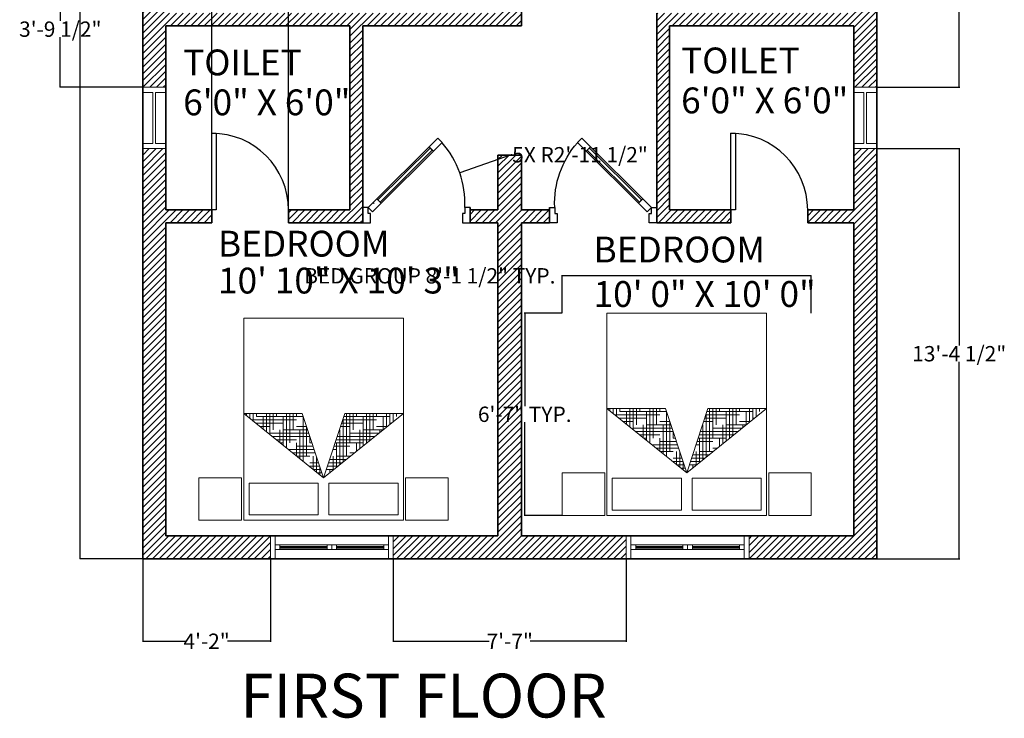
# Model space of a CAD drawing. Units: inches. Extents: x 585 to 1401, y -184 to 463.
# Tile 7 of 8: x 1016 to 1401, y -172 to 101. Entities that reach past the tile are written whole.
import ezdxf

# ---------------------------------------------------------------- set-up
doc = ezdxf.new("R2010")
doc.units = ezdxf.units.IN
doc.header["$MEASUREMENT"] = 0
for name, color, linetype, lineweight in [('A-ANNO-DIMS', 2, 'Continuous', 18), ('A-ANNO-TEXT', 7, 'Continuous', 25), ('A-AREA-IDEN', 7, 'Continuous', 18), ('A-Door', 150, 'Continuous', 25), ('A-FURN', 8, 'Continuous', 18), ('A-Glaz', 140, 'Continuous', 18), ('A-Wall', 7, 'Continuous', 35), ('A-WALL-PATT', 252, 'Continuous', 13)]:
    doc.layers.add(name, color=color, linetype=linetype, lineweight=lineweight)
doc.styles.get("Standard").update_dxf_attribs({"font": 'arial.ttf'})
doc.dimstyles.get("Standard").update_dxf_attribs({"dimtxt": 6, "dimasz": 0.18, "dimexe": 0.18, "dimexo": 0.0625, "dimgap": 0.09, "dimtad": 0, "dimtih": 1, "dimtoh": 1, "dimdec": 0, "dimzin": 0, "dimdsep": 46, "dimlunit": 3, "dimtxsty": 'Standard', "dimblk": 'ARCHTICK', "dimcen": 0.09, "dimadec": 0, "dimazin": 0, "dimtfac": 1, "dimtdec": 0, "dimtofl": 0, "dimtmove": 0, "dimatfit": 3, "dimfxl": 1, "dimtolj": 1, "dimtzin": 0, "dimarcsym": 0})

# ---------------------------------------------------------------- blocks, each defined once
blk = doc.blocks.new('A$C1DF4181C')
blk.add_lwpolyline([(120, 128), (460.7, 466.1), (432.5, 494.5), (91.8, 156.4)], close=True)
blk.add_arc((72.4, 128.7), 593.3, 357.23132, 41.49368)
at = {"layer": 'A-Door'}
for points in [[(517.5, 522.4), (460.7, 466.1), (432.5, 494.5), (489.3, 550.8)], [(63.2, 71.6), (120, 128), (91.8, 156.4), (35, 100)], [(35, 100), (0, 100), (0, 0), (50, 0), (50, 50), (50, 60), (35, 60)], [(665, 100), (665, 60), (650, 60), (650, 50), (650, 0), (700, 0), (700, 100)]]:
    blk.add_lwpolyline(points, close=True, dxfattribs=at)
at = {"layer": 'A-Glaz'}
blk.add_lwpolyline([(112.9, 135.1), (453.6, 473.2), (439.5, 487.4), (98.8, 149.3)], close=True, dxfattribs=at)
at = {"layer": 'A-Wall'}
for p, q in [((0, 0), (0, 100)), ((0, 100), (0, 0)), ((700, 0), (700, 100)), ((700, 0), (700, 100))]:
    blk.add_line(p, q, dxfattribs=at)
blk = doc.blocks.new('*U9')
for p, q in [((0, 0), (0, -5)), ((30, 0), (30, -5))]:
    blk.add_line(p, q)
blk.add_lwpolyline([(0, 0), (0, 30), (1.75, 30), (1.75, 0)], close=True)
blk.add_arc((0, 0), 30, 0, 90)
blk = doc.blocks.new('*X23')
at = {"color": 0}
for p, q in [((20.25, 14.8125), (20.2772, 14.8125)), ((20.1487, 14.7188), (20.2772, 14.7188)), ((20.1562, 14.625), (20.1562, 14.7281)), ((20.1739, 14.75), (20.2772, 14.75)), ((20.1875, 14.75), (20.1875, 14.7669)), ((20.199, 14.7812), (20.2772, 14.7812)), ((20.25, 14.3194), (20.25, 14.75)), ((20.0625, 14.2573), (20.0625, 14.6116)), ((20.0938, 14.375), (20.0938, 14.6504)), ((20.0984, 14.6562), (20.125, 14.6562)), ((20.1236, 14.6875), (20.25, 14.6875)), ((20.125, 14.5), (20.125, 14.6893)), ((20.2188, 14.3091), (20.2188, 14.625)), ((20.25, 14.625), (20.2772, 14.625)), ((19.9979, 14.5312), (20.2772, 14.5312)), ((20.023, 14.5625), (20.2772, 14.5625)), ((20.0312, 14.2469), (20.0312, 14.5727)), ((20.125, 14.5938), (20.2772, 14.5938)), ((19.9225, 14.4375), (20, 14.4375)), ((19.9476, 14.4688), (20.125, 14.4688)), ((19.9727, 14.5), (20.25, 14.5)), ((20, 14.2366), (20, 14.5)), ((20.1875, 14.2987), (20.1875, 14.5)), ((20.25, 14.4375), (20.2772, 14.4375)), ((19.8438, 14.1848), (19.8438, 14.3397)), ((19.875, 14.25), (19.875, 14.3785)), ((19.875, 14.3438), (20.2772, 14.3438)), ((19.9062, 14.375), (19.9062, 14.4174)), ((19.9688, 14.2262), (19.9688, 14.375)), ((20, 14.375), (20.2772, 14.375)), ((20.125, 14.4062), (20.2772, 14.4062)), ((20.1562, 14.2884), (20.1562, 14.375)), ((19.7716, 14.25), (20, 14.25)), ((19.7812, 14.1641), (19.7812, 14.262)), ((19.7967, 14.2812), (20.125, 14.2812)), ((19.8125, 14.1744), (19.8125, 14.3008)), ((19.8219, 14.3125), (20.2291, 14.3125)), ((19.9375, 14.2159), (19.9375, 14.25)), ((19.7213, 14.1875), (19.75, 14.1875)), ((19.7465, 14.2188), (19.875, 14.2188)), ((19.75, 14.1537), (19.75, 14.2231)), ((19.7018, 14.0938), (19.7786, 14.0938)), ((19.7188, 14.0726), (19.7188, 14.1136)), ((19.7269, 14.0625), (19.8728, 14.0625)), ((19.75, 14.0338), (19.75, 14.1032)), ((19.7812, 13.9949), (19.7812, 14.0929)), ((19.8125, 14), (19.8125, 14.0825)), ((19.752, 14.0312), (19.875, 14.0312)), ((19.875, 13.8784), (19.875, 14)), ((19.875, 13.9688), (20.1557, 13.9688)), ((19.9062, 13.8396), (19.9062, 14.0514)), ((19.9375, 13.8007), (19.9375, 14.0411)), ((19.9688, 13.875), (19.9688, 14.0307)), ((20, 14), (20, 14.0204)), ((20, 14), (20.0614, 14)), ((20.0625, 13.6454), (20.0625, 13.9996)), ((20.0938, 13.625), (20.0938, 13.9893)), ((20.125, 13.75), (20.125, 13.9789)), ((20.1562, 13.875), (20.1562, 13.9686)), ((19.8275, 13.9375), (20.25, 13.9375)), ((19.8526, 13.9062), (20.125, 13.9062)), ((19.8777, 13.875), (20, 13.875)), ((20.0312, 13.6842), (20.0312, 13.875)), ((20.2188, 13.4511), (20.2188, 13.875)), ((20.25, 13.5), (20.25, 13.9375)), ((20.25, 13.875), (20.2772, 13.875)), ((19.9532, 13.7812), (20.2772, 13.7812)), ((20, 13.8125), (20.2772, 13.8125)), ((20.125, 13.8438), (20.2772, 13.8438)), ((19.9783, 13.75), (20.25, 13.75)), ((20, 13.723), (20, 13.75)), ((20.0035, 13.7188), (20.125, 13.7188)), ((20.1875, 13.49), (20.1875, 13.75)), ((20.25, 13.6875), (20.2772, 13.6875)), ((20.0789, 13.625), (20.2772, 13.625)), ((20.104, 13.5938), (20.2772, 13.5938)), ((20.125, 13.6562), (20.2772, 13.6562)), ((20.1562, 13.5288), (20.1562, 13.625)), ((20.1292, 13.5625), (20.25, 13.5625)), ((20.2046, 13.4688), (20.2772, 13.4688)), ((20.2297, 13.4375), (20.2772, 13.4375)), ((20.25, 13.5), (20.2772, 13.5)), ((20.2549, 13.4062), (20.2772, 13.4062))]:
    blk.add_line(p, q, dxfattribs=at)
blk = doc.blocks.new('MAT-P02')
for p, q in [((-1.17, 0), (-1.17, -0.4)), ((-1.17, 0), (-0.77, 0)), ((-0.77, 0), (-0.77, -0.4)), ((-0.75, 0), (0.75, 0)), ((-0.75, 0), (-0.75, -1.9)), ((0.75, 0), (0.75, -1.9)), ((0.77, 0), (1.17, 0)), ((0.77, 0), (0.77, -0.4)), ((1.17, 0), (1.17, -0.4)), ((-0.7, -0.05), (-0.7, -0.35)), ((-0.7, -0.05), (-0.05, -0.05)), ((-0.05, -0.35), (-0.05, -0.05)), ((0.05, -0.05), (0.7, -0.05)), ((0.05, -0.35), (0.05, -0.05)), ((0.7, -0.05), (0.7, -0.35)), ((-0.7, -0.35), (-0.05, -0.35)), ((0.05, -0.35), (0.7, -0.35)), ((-1.17, -0.4), (-0.77, -0.4)), ((-0.75, -1.0034), (0, -0.4)), ((0, -0.4), (-0.75, -1.0034)), ((0, -0.4), (-0.2, -1.0034)), ((0, -0.4), (0.2, -1.0034)), ((0, -0.4), (0.75, -1.0034)), ((0.77, -0.4), (1.17, -0.4)), ((-0.75, -1.0034), (-0.2, -1.0034)), ((0.2, -1.0034), (0.75, -1.0034)), ((0.75, -1.9), (-0.75, -1.9))]:
    blk.add_line(p, q)
at = {"xscale": -1, "rotation": 90}
blk.add_blockref('*X23', (14.1285, 19.2738), dxfattribs=at)
blk = doc.blocks.new('_ArchTick')
at = {"color": 0, "linetype": 'ByBlock', "const_width": 0.15}
blk.add_lwpolyline([(-0.5, -0.5), (0.5, 0.5)], dxfattribs=at)
blk = doc.blocks.new('*D30')
at = {"layer": 'A-ANNO-DIMS', "color": 0, "lineweight": -2, "transparency": 16777216}
for p, q in [((1064.47, 422.15), (1039.92, 422.15)), ((1040.1, 422.15), (1040.1, 159.24)), ((1040.1, -109.85), (1040.1, 153.06)), ((1064.47, -109.85), (1039.92, -109.85))]:
    blk.add_line(p, q, dxfattribs=at)
at = {"layer": 'Defpoints', "color": 0, "transparency": 16777216}
for p in [(1064.54, 422.15), (1040.1, -109.85), (1064.54, -109.85)]:
    blk.add_point(p, dxfattribs=at)
at = {"layer": 'A-ANNO-DIMS', "color": 0, "lineweight": -2, "transparency": 16777216, "xscale": 0.18, "yscale": 0.18, "zscale": 0.18}
for p, rotation in [((1040.1, 422.15), 90), ((1040.1, -109.85), 270)]:
    blk.add_blockref('_ArchTick', p, dxfattribs=dict(at, rotation=rotation))
at = {"layer": 'A-ANNO-DIMS', "color": 0, "transparency": 16777216, "insert": (1040.1, 156.15), "char_height": 6, "attachment_point": 5}
blk.add_mtext('\\A1;44\'-4"', dxfattribs=at)
blk = doc.blocks.new('WIN-48-DOUBLE-PANEL')
for p, q in [((48, 9), (0, 9)), ((0, 9), (0, 0)), ((1.85, 9), (0, 9)), ((0, 9), (0, 0)), ((1.85, 0), (1.85, 9)), ((1.85, 0), (1.85, 9)), ((46.15, 9), (48, 9)), ((46.15, 0), (46.15, 9)), ((46.15, 0), (46.15, 9)), ((46.15, 0), (46.15, 9)), ((48, 9), (48, 0)), ((48, 0), (48, 9)), ((1.85, 5.44), (46.15, 5.44)), ((3.69, 3.6), (3.69, 5.44)), ((3.69, 4.89), (22.15, 4.89)), ((3.69, 4.52), (22.15, 4.52)), ((3.69, 4.15), (22.15, 4.15)), ((22.15, 5.44), (22.15, 3.6)), ((24, 5.44), (24, 3.6)), ((25.85, 5.44), (25.85, 3.6)), ((44.31, 4.89), (25.85, 4.89)), ((44.31, 4.52), (25.85, 4.52)), ((44.31, 4.15), (25.85, 4.15)), ((44.31, 3.6), (44.31, 5.44)), ((0, 0), (1.85, 0)), ((48, 0), (0, 0)), ((1.85, 3.6), (46.15, 3.6)), ((48, 0), (46.15, 0))]:
    blk.add_line(p, q)
blk = doc.blocks.new('WIN-24-SINGLE-PANEL')
for p, q in [((0, 0), (0, 24)), ((0, 24), (9, 24)), ((9, 24), (9, 0)), ((0, 22), (4, 22)), ((4, 22), (4, 2)), ((5, 22), (9, 22)), ((5, 22), (5, 2)), ((4, 2), (0, 2)), ((9, 0), (0, 0)), ((9, 2), (5, 2))]:
    blk.add_line(p, q)
blk = doc.blocks.new('*D46')
at = {"layer": 'A-ANNO-DIMS', "color": 0, "lineweight": -2, "transparency": 16777216}
for p, q in [((1228.51, 0.88), (1228.33, 0.88)), ((1228.51, -13.68), (1228.51, 1.06)), ((1325.94, 0.88), (1228.51, 0.88)), ((1325.94, -13.68), (1325.94, 1.06))]:
    blk.add_line(p, q, dxfattribs=at)
at = {"layer": 'Defpoints', "color": 0, "transparency": 16777216}
for p in [(1228.51, 0.88), (1228.51, -13.74), (1325.94, -13.74)]:
    blk.add_point(p, dxfattribs=at)
at = {"layer": 'A-ANNO-DIMS', "color": 0, "lineweight": -2, "transparency": 16777216, "xscale": 0.18, "yscale": 0.18, "zscale": 0.18, "rotation": 180}
blk.add_blockref('_ArchTick', (1228.51, 0.88), dxfattribs=at)
at = {"layer": 'A-ANNO-DIMS', "color": 0, "lineweight": -2, "transparency": 16777216, "xscale": 0.18, "yscale": 0.18, "zscale": 0.18}
blk.add_blockref('_ArchTick', (1325.94, 0.88), dxfattribs=at)
at = {"layer": 'A-ANNO-DIMS', "color": 0, "transparency": 16777216, "insert": (1176.78, 0.88), "char_height": 6, "attachment_point": 5}
blk.add_mtext('\\A1;BED GROUP 8\'-1 1/2" TYP.', dxfattribs=at)
blk = doc.blocks.new('*D47')
at = {"layer": 'A-ANNO-DIMS', "color": 0, "lineweight": -2, "transparency": 16777216}
for p, q in [((1228.45, -13.74), (1213.72, -13.74)), ((1213.9, -13.74), (1213.9, -50.14)), ((1213.9, -92.84), (1213.9, -56.44)), ((1228.45, -92.84), (1213.72, -92.84))]:
    blk.add_line(p, q, dxfattribs=at)
at = {"layer": 'Defpoints', "color": 0, "transparency": 16777216}
for p in [(1228.51, -13.74), (1213.9, -92.84), (1228.51, -92.84)]:
    blk.add_point(p, dxfattribs=at)
at = {"layer": 'A-ANNO-DIMS', "color": 0, "lineweight": -2, "transparency": 16777216, "xscale": 0.18, "yscale": 0.18, "zscale": 0.18}
for p, rotation in [((1213.9, -13.74), 90), ((1213.9, -92.84), 270)]:
    blk.add_blockref('_ArchTick', p, dxfattribs=dict(at, rotation=rotation))
at = {"layer": 'A-ANNO-DIMS', "color": 0, "transparency": 16777216, "insert": (1213.9, -53.29), "char_height": 6, "attachment_point": 5}
blk.add_mtext('\\A1;6\'-7" TYP.', dxfattribs=at)
blk = doc.blocks.new('*D90')
at = {"layer": 'A-ANNO-DIMS', "color": 0, "lineweight": -2, "transparency": 16777216}
for p, q in [((1064.54, -109.91), (1064.54, -142.28)), ((1114.49, -109.91), (1114.49, -142.28)), ((1064.54, -142.1), (1081.33, -142.1)), ((1114.49, -142.1), (1097.7, -142.1))]:
    blk.add_line(p, q, dxfattribs=at)
at = {"layer": 'Defpoints', "color": 0, "transparency": 16777216}
for p in [(1064.54, -109.85), (1114.49, -109.85), (1114.49, -142.1)]:
    blk.add_point(p, dxfattribs=at)
at = {"layer": 'A-ANNO-DIMS', "color": 0, "lineweight": -2, "transparency": 16777216, "xscale": 0.18, "yscale": 0.18, "zscale": 0.18, "rotation": 180}
blk.add_blockref('_ArchTick', (1064.54, -142.1), dxfattribs=at)
at = {"layer": 'A-ANNO-DIMS', "color": 0, "lineweight": -2, "transparency": 16777216, "xscale": 0.18, "yscale": 0.18, "zscale": 0.18}
blk.add_blockref('_ArchTick', (1114.49, -142.1), dxfattribs=at)
at = {"layer": 'A-ANNO-DIMS', "color": 0, "transparency": 16777216, "insert": (1089.51, -142.1), "char_height": 6, "attachment_point": 5}
blk.add_mtext('\\A1;4\'-2"', dxfattribs=at)
blk = doc.blocks.new('*D91')
at = {"layer": 'A-ANNO-DIMS', "color": 0, "lineweight": -2, "transparency": 16777216}
for p, q in [((1162.49, -109.91), (1162.49, -142.28)), ((1253.59, -109.91), (1253.59, -142.28)), ((1162.49, -142.1), (1200, -142.1)), ((1253.59, -142.1), (1216.08, -142.1))]:
    blk.add_line(p, q, dxfattribs=at)
at = {"layer": 'Defpoints', "color": 0, "transparency": 16777216}
for p in [(1162.49, -109.85), (1253.59, -109.85), (1253.59, -142.1)]:
    blk.add_point(p, dxfattribs=at)
at = {"layer": 'A-ANNO-DIMS', "color": 0, "lineweight": -2, "transparency": 16777216, "xscale": 0.18, "yscale": 0.18, "zscale": 0.18, "rotation": 180}
blk.add_blockref('_ArchTick', (1162.49, -142.1), dxfattribs=at)
at = {"layer": 'A-ANNO-DIMS', "color": 0, "lineweight": -2, "transparency": 16777216, "xscale": 0.18, "yscale": 0.18, "zscale": 0.18}
blk.add_blockref('_ArchTick', (1253.59, -142.1), dxfattribs=at)
at = {"layer": 'A-ANNO-DIMS', "color": 0, "transparency": 16777216, "insert": (1208.04, -142.1), "char_height": 6, "attachment_point": 5}
blk.add_mtext('\\A1;7\'-7"', dxfattribs=at)
blk = doc.blocks.new('*D92')
at = {"layer": 'A-ANNO-DIMS', "color": 0, "lineweight": -2, "transparency": 16777216}
for p, q in [((1351.6, 50.65), (1383.97, 50.65)), ((1383.79, 50.65), (1383.79, -26.4)), ((1383.79, -109.85), (1383.79, -32.79)), ((1351.6, -109.85), (1383.97, -109.85))]:
    blk.add_line(p, q, dxfattribs=at)
at = {"layer": 'Defpoints', "color": 0, "transparency": 16777216}
for p in [(1351.54, 50.65), (1383.79, 50.65), (1351.54, -109.85)]:
    blk.add_point(p, dxfattribs=at)
at = {"layer": 'A-ANNO-DIMS', "color": 0, "lineweight": -2, "transparency": 16777216, "xscale": 0.18, "yscale": 0.18, "zscale": 0.18}
for p, rotation in [((1383.79, 50.65), 90), ((1383.79, -109.85), 270)]:
    blk.add_blockref('_ArchTick', p, dxfattribs=dict(at, rotation=rotation))
at = {"layer": 'A-ANNO-DIMS', "color": 0, "transparency": 16777216, "insert": (1383.79, -29.6), "char_height": 6, "attachment_point": 5}
blk.add_mtext('\\A1;13\'-4 1/2"', dxfattribs=at)
blk = doc.blocks.new('*D93')
at = {"layer": 'A-ANNO-DIMS', "color": 0, "lineweight": -2, "transparency": 16777216}
for p, q in [((1351.6, 183.9), (1383.97, 183.9)), ((1383.79, 183.9), (1383.79, 132.47)), ((1383.79, 74.65), (1383.79, 126.09)), ((1351.6, 74.65), (1383.97, 74.65))]:
    blk.add_line(p, q, dxfattribs=at)
at = {"layer": 'Defpoints', "color": 0, "transparency": 16777216}
for p in [(1351.54, 183.9), (1383.79, 183.9), (1351.54, 74.65)]:
    blk.add_point(p, dxfattribs=at)
at = {"layer": 'A-ANNO-DIMS', "color": 0, "lineweight": -2, "transparency": 16777216, "xscale": 0.18, "yscale": 0.18, "zscale": 0.18}
for p, rotation in [((1383.79, 183.9), 90), ((1383.79, 74.65), 270)]:
    blk.add_blockref('_ArchTick', p, dxfattribs=dict(at, rotation=rotation))
at = {"layer": 'A-ANNO-DIMS', "color": 0, "transparency": 16777216, "insert": (1383.79, 129.28), "char_height": 6, "attachment_point": 5}
blk.add_mtext('\\A1;9\'-1 1/2"', dxfattribs=at)
blk = doc.blocks.new('*D94')
at = {"layer": 'A-ANNO-DIMS', "color": 0, "lineweight": -2, "transparency": 16777216}
for p, q in [((1064.47, 120.15), (1032.11, 120.15)), ((1032.29, 120.15), (1032.29, 100.6)), ((1032.29, 74.65), (1032.29, 94.21)), ((1064.47, 74.65), (1032.11, 74.65))]:
    blk.add_line(p, q, dxfattribs=at)
at = {"layer": 'Defpoints', "color": 0, "transparency": 16777216}
for p in [(1032.29, 120.15), (1064.54, 120.15), (1064.54, 74.65)]:
    blk.add_point(p, dxfattribs=at)
at = {"layer": 'A-ANNO-DIMS', "color": 0, "lineweight": -2, "transparency": 16777216, "xscale": 0.18, "yscale": 0.18, "zscale": 0.18}
for p, rotation in [((1032.29, 120.15), 90), ((1032.29, 74.65), 270)]:
    blk.add_blockref('_ArchTick', p, dxfattribs=dict(at, rotation=rotation))
at = {"layer": 'A-ANNO-DIMS', "color": 0, "transparency": 16777216, "insert": (1032.29, 97.4), "char_height": 6, "attachment_point": 5}
blk.add_mtext('\\A1;3\'-9 1/2"', dxfattribs=at)
blk = doc.blocks.new('*D95')
at = {"layer": 'A-ANNO-DIMS', "color": 0, "lineweight": -2, "transparency": 16777216}
for p, q in [((1091.54, 26.72), (1091.54, 454.58)), ((1091.54, 454.4), (1098.42, 454.4)), ((1121.54, 454.4), (1114.65, 454.4)), ((1121.54, 26.72), (1121.54, 454.58))]:
    blk.add_line(p, q, dxfattribs=at)
at = {"layer": 'Defpoints', "color": 0, "transparency": 16777216}
for p in [(1121.54, 454.4), (1091.54, 26.65), (1121.54, 26.65)]:
    blk.add_point(p, dxfattribs=at)
at = {"layer": 'A-ANNO-DIMS', "color": 0, "lineweight": -2, "transparency": 16777216, "xscale": 0.18, "yscale": 0.18, "zscale": 0.18, "rotation": 180}
blk.add_blockref('_ArchTick', (1091.54, 454.4), dxfattribs=at)
at = {"layer": 'A-ANNO-DIMS', "color": 0, "lineweight": -2, "transparency": 16777216, "xscale": 0.18, "yscale": 0.18, "zscale": 0.18}
blk.add_blockref('_ArchTick', (1121.54, 454.4), dxfattribs=at)
at = {"layer": 'A-ANNO-DIMS', "color": 0, "transparency": 16777216, "insert": (1106.54, 454.4), "char_height": 6, "attachment_point": 5}
blk.add_mtext('\\A1;2\'-6"', dxfattribs=at)
blk = doc.blocks.new('*D96')
at = {"layer": 'A-ANNO-DIMS', "color": 0, "lineweight": -2, "transparency": 16777216}
for p, q in [((1208.62, 48.26), (1188.46, 41.17)), ((1208.8, 48.26), (1208.62, 48.26)), ((1154.79, 29.37), (1154.97, 29.37)), ((1154.88, 29.28), (1154.88, 29.46))]:
    blk.add_line(p, q, dxfattribs=at)
at = {"layer": 'Defpoints', "color": 0, "transparency": 16777216}
for p in [(1188.46, 41.17), (1154.88, 29.37)]:
    blk.add_point(p, dxfattribs=at)
at = {"layer": 'A-ANNO-DIMS', "color": 0, "lineweight": -2, "transparency": 16777216, "xscale": 0.18, "yscale": 0.18, "zscale": 0.18, "rotation": 199.3624875231046}
blk.add_blockref('_ArchTick', (1188.46, 41.17), dxfattribs=at)
at = {"layer": 'A-ANNO-DIMS', "color": 0, "transparency": 16777216, "insert": (1235.5, 48.26), "char_height": 6, "attachment_point": 5}
blk.add_mtext('\\A1;5X R2\'-11 1/2"', dxfattribs=at)

msp = doc.modelspace()

# ---------------------------------------------------------------- hatches: boundary and pattern name
at = {"layer": 'A-WALL-PATT'}
h = msp.add_hatch(dxfattribs=at)
h.set_pattern_fill('ANSI31', color=256, scale=15)
h.set_pattern_definition([(45, (64.5137, -1e-14), (-1.3258252, 1.3258252), [])])
h.paths.add_polyline_path([(1351.54, 50.65), (1342.54, 50.65), (1342.54, 26.65), (1324.54, 26.65), (1324.54, 21.65), (1342.54, 21.65), (1342.54, -100.85), (1301.59, -100.85), (1301.59, -109.85), (1351.54, -109.85)])
h.paths.add_polyline_path([(1351.54, 183.9), (1342.54, 183.9), (1342.54, 103.65), (1265.54, 103.65), (1265.54, 26.65), (1265.54, 21.65), (1270.54, 21.65), (1294.54, 21.65), (1294.54, 26.65), (1270.54, 26.65), (1270.54, 98.65), (1342.54, 98.65), (1342.54, 74.65), (1351.54, 74.65)])
h.paths.add_polyline_path([(1212.64, 117.9), (1203.44, 117.9), (1203.44, 103.65), (1145.54, 103.65), (1073.54, 103.65), (1073.54, 120.15), (1064.54, 120.15), (1064.54, 74.65), (1073.54, 74.65), (1073.54, 98.65), (1145.54, 98.65), (1145.54, 26.65), (1121.54, 26.65), (1121.54, 21.65), (1145.54, 21.65), (1150.54, 21.65), (1150.54, 26.65), (1150.54, 98.65), (1212.64, 98.65)])
h.paths.add_polyline_path([(1073.54, 21.65), (1091.54, 21.65), (1091.54, 26.65), (1073.54, 26.65), (1073.54, 50.65), (1064.54, 50.65), (1064.54, -109.85), (1114.49, -109.85), (1114.49, -100.85), (1073.54, -100.85)])
h.paths.add_polyline_path([(1253.59, -100.85), (1212.64, -100.85), (1212.64, 21.65), (1223.54, 21.65), (1223.54, 26.65), (1212.64, 26.65), (1212.64, 43.15), (1212.64, 48.15), (1203.44, 48.15), (1203.44, 43.15), (1203.44, 26.65), (1192.54, 26.65), (1192.54, 21.65), (1203.44, 21.65), (1203.44, -100.85), (1162.49, -100.85), (1162.49, -109.85), (1163.54, -109.85), (1253.59, -109.85)])
h.paths.add_polyline_path([(1073.54, 264.15), (1222.54, 264.15), (1222.54, 269.15), (1073.54, 269.15), (1073.54, 413.15), (1121.54, 413.15), (1121.54, 422.15), (1064.54, 422.15), (1064.54, 168.15), (1073.54, 168.15), (1073.54, 185.15), (1203.44, 185.15), (1203.44, 153.9), (1212.64, 153.9), (1212.64, 185.15), (1222.54, 185.15), (1222.54, 190.15), (1073.54, 190.15)])
h.paths.add_polyline_path([(1258.54, 422.15), (1169.54, 422.15), (1169.54, 413.15), (1217.54, 413.15), (1217.54, 312.15), (1258.54, 312.15), (1258.54, 317.15), (1222.54, 317.15), (1222.54, 413.15), (1258.54, 413.15)])
h.paths.add_polyline_path([(1351.54, 422.15), (1306.54, 422.15), (1306.54, 413.15), (1342.54, 413.15), (1342.54, 317.15), (1306.54, 317.15), (1306.54, 312.15), (1342.54, 312.15), (1342.54, 231.9), (1351.54, 231.9)])

# ---------------------------------------------------------------- linework, layer by layer
at = {"layer": 'A-Wall'}
for p, q in [((1064.54, 422.15), (1064.54, -109.85)), ((1351.54, 422.15), (1351.54, -109.85)), ((1212.64, 98.65), (1212.64, 117.9)), ((1265.54, 103.65), (1265.54, 26.65)), ((1073.54, 98.65), (1145.54, 98.65)), ((1073.54, 98.65), (1073.54, 26.65)), ((1145.54, 98.65), (1145.54, 26.65)), ((1150.54, 98.65), (1150.54, 26.65)), ((1150.54, 98.65), (1212.64, 98.65)), ((1270.54, 98.65), (1270.54, 26.65)), ((1270.54, 98.65), (1342.54, 98.65)), ((1342.54, 98.65), (1342.54, 26.65)), ((1203.44, 48.15), (1212.64, 48.15)), ((1203.44, 43.15), (1203.44, 48.15)), ((1212.64, 48.15), (1203.44, 48.15)), ((1212.64, 43.15), (1212.64, 48.15)), ((1212.64, 26.65), (1212.64, 48.15)), ((1203.44, 26.65), (1203.44, 43.15)), ((1212.64, 26.65), (1212.64, 43.15)), ((1342.54, 43.15), (1342.54, 26.65)), ((1073.54, 26.65), (1091.54, 26.65)), ((1091.54, 26.65), (1091.54, 21.65)), ((1121.54, 26.65), (1121.54, 21.65)), ((1121.54, 26.65), (1145.54, 26.65)), ((1150.54, 26.65), (1150.54, 21.65)), ((1192.54, 26.65), (1203.44, 26.65)), ((1192.54, 26.65), (1192.54, 21.65)), ((1223.54, 26.65), (1212.64, 26.65)), ((1223.54, 26.65), (1223.54, 21.65)), ((1265.54, 26.65), (1265.54, 21.65)), ((1294.54, 26.65), (1270.54, 26.65)), ((1294.54, 26.65), (1294.54, 21.65)), ((1342.54, 26.65), (1324.54, 26.65)), ((1324.54, 26.65), (1324.54, 21.65)), ((1073.54, 21.65), (1091.54, 21.65)), ((1073.54, 21.65), (1073.54, -100.85)), ((1121.54, 21.65), (1145.54, 21.65)), ((1145.54, 21.65), (1150.54, 21.65)), ((1192.54, 21.65), (1203.44, 21.65)), ((1203.44, -100.85), (1203.44, 21.65)), ((1212.64, -100.85), (1212.64, 21.65)), ((1212.64, -100.85), (1212.64, 21.65)), ((1223.54, 21.65), (1212.64, 21.65)), ((1270.54, 21.65), (1265.54, 21.65)), ((1294.54, 21.65), (1270.54, 21.65)), ((1342.54, 21.65), (1324.54, 21.65)), ((1342.54, 21.65), (1342.54, -100.85)), ((1073.54, -100.85), (1203.44, -100.85)), ((1212.64, -100.85), (1342.54, -100.85)), ((1064.54, -109.85), (1163.54, -109.85)), ((1163.54, -109.85), (1351.54, -109.85))]:
    msp.add_line(p, q, dxfattribs=at)

# ---------------------------------------------------------------- block references
at = {"layer": 'A-Door'}
for p in [(1091.54, 26.65), (1294.54, 26.65)]:
    msp.add_blockref('*U9', p, dxfattribs=at)
at = {"layer": 'A-Door', "yscale": 0.0599999999683043, "zscale": 0.0599999999683043}
for p, xscale in [((1150.54, 21.65), 0.0599999999683043), ((1265.54, 21.65), -0.0599999999683043)]:
    msp.add_blockref('A$C1DF4181C', p, dxfattribs=dict(at, xscale=xscale))
at = {"layer": 'A-FURN', "xscale": 41.63451012544946, "yscale": 41.63451012544946, "zscale": 41.63451012544946, "rotation": 180}
for p in [(1277.23, -92.84), (1135.23, -94.76)]:
    msp.add_blockref('MAT-P02', p, dxfattribs=at)
at = {"layer": 'A-Glaz', "rotation": 180}
for p in [(1073.54, 74.65), (1351.54, 74.65)]:
    msp.add_blockref('WIN-24-SINGLE-PANEL', p, dxfattribs=at)
at = {"layer": 'A-Glaz'}
for p in [(1114.49, -109.85), (1253.59, -109.85)]:
    msp.add_blockref('WIN-48-DOUBLE-PANEL', p, dxfattribs=at)

# ---------------------------------------------------------------- texts
at = {"layer": 'A-ANNO-TEXT'}
msp.add_text('FIRST FLOOR', height=17.1732, dxfattribs=at).set_placement((1102.72, -171.95))
at = {"layer": 'A-AREA-IDEN'}
for s, height, p in [('TOILET', 10.101, (1080.35, 79.33)), ('TOILET', 10.101, (1275.05, 80.09)), ('6\'0" X 6\'0"', 10.1013, (1080.35, 63.7)), ('6\'0" X 6\'0"', 10.1013, (1275.05, 64.46)), ('BEDROOM', 10.101, (1093.96, 8.41)), ('BEDROOM', 10.101, (1240.82, 6.12)), ('10\' 10" X 10\' 3"', 10.1013, (1093.96, -6.03)), ('10\' 0" X 10\' 0"', 10.1013, (1240.82, -11.28))]:
    msp.add_text(s, height=height, dxfattribs=at).set_placement(p)

# ---------------------------------------------------------------- dimensions: what is measured, and where the dimension line sits
at = {"layer": 'A-ANNO-DIMS'}
for base, p1, p2, picture, middle in [((1121.54, 454.4), (1091.54, 26.65), (1121.54, 26.65), '*D95', (1106.54, 454.4)), ((1114.486878, -142.096921), (1064.536878, -109.846921), (1114.486878, -109.846921), '*D90', (1089.511878, -142.096921)), ((1253.59, -142.1), (1162.49, -109.85), (1253.59, -109.85), '*D91', (1208.04, -142.1))]:
    dim = msp.add_linear_dim(base=base, p1=p1, p2=p2, dimstyle='Standard', override={"dimdec": 1, "dimlfac": 1, "dimrnd": 0, "dimzin": 1, "dimdsep": 46, "dimlunit": 4, "dimfrac": 2}, dxfattribs=at)
    dim.commit()
    dim.dimension.update_dxf_attribs({"geometry": picture, "text_midpoint": middle})
for base, p1, p2, override, picture, middle in [((1040.1, -109.85), (1064.54, 422.15), (1064.54, -109.85), {"dimclrd": 0, "dimclre": 0, "dimclrt": 0}, '*D30', (1040.1, 156.15)), ((1383.786878, 183.903079), (1351.536878, 74.653079), (1351.536878, 183.903079), {"dimdec": 1, "dimlfac": 1, "dimrnd": 0, "dimzin": 1, "dimdsep": 46, "dimlunit": 4, "dimfrac": 2}, '*D93', (1383.786878, 129.278079)), ((1032.29, 120.15), (1064.54, 74.65), (1064.54, 120.15), {"dimdec": 1, "dimlfac": 1, "dimrnd": 0, "dimzin": 1, "dimdsep": 46, "dimlunit": 4, "dimfrac": 2}, '*D94', (1032.29, 97.4)), ((1383.79, 50.65), (1351.54, -109.85), (1351.54, 50.65), {"dimdec": 1, "dimlfac": 1, "dimrnd": 0, "dimzin": 1, "dimdsep": 46, "dimlunit": 4, "dimfrac": 2}, '*D92', (1383.79, -29.6))]:
    dim = msp.add_linear_dim(base=base, p1=p1, p2=p2, angle=90, dimstyle='Standard', override=override, dxfattribs=at)
    dim.commit()
    dim.dimension.update_dxf_attribs({"geometry": picture, "text_midpoint": middle})
dim = msp.add_radius_dim(center=(1154.88, 29.37), mpoint=(1188.46, 41.17), text='5X <>', dimstyle='Standard', override={"dimdec": 1, "dimlfac": 1, "dimrnd": 0, "dimzin": 1, "dimdsep": 46, "dimlunit": 4, "dimfrac": 2}, dxfattribs=at)
dim.commit()
dim.dimension.update_dxf_attribs({"geometry": '*D96', "text_midpoint": (1235.5, 48.26), "dimtype": 164})
for base, p1, p2, angle, text, picture, middle in [((1228.51, 0.88), (1325.94, -13.74), (1228.51, -13.74), 180, 'BED GROUP <> TYP.', '*D46', (1176.78, 0.88)), ((1213.9, -92.84), (1228.51, -13.74), (1228.51, -92.84), 270, '<> TYP.', '*D47', (1213.9, -53.29))]:
    dim = msp.add_linear_dim(base=base, p1=p1, p2=p2, angle=angle, text=text, dimstyle='Standard', override={"dimdec": 1, "dimlfac": 1, "dimrnd": 0, "dimzin": 1, "dimdsep": 46, "dimlunit": 4, "dimfrac": 2}, dxfattribs=at)
    dim.commit()
    dim.dimension.update_dxf_attribs({"geometry": picture, "text_midpoint": middle})

doc.saveas('drawing.dxf')
